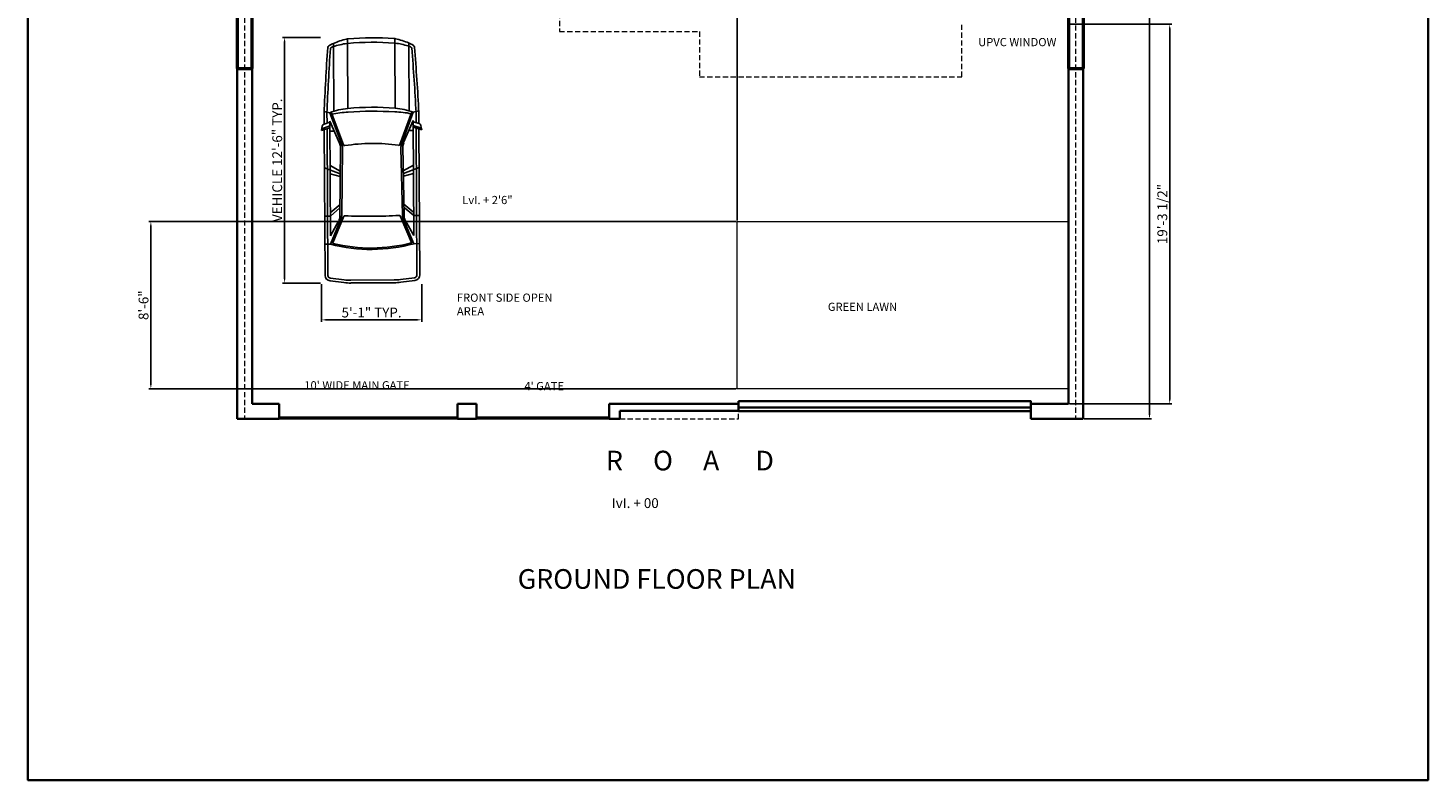
# Model space of a CAD drawing. Units: inches. Extents: x 2123 to 2977, y 1464 to 2698.
# Tile 1 of 10: x 2123 to 2977, y 1464 to 1923. Entities that reach past the tile are written whole.
import ezdxf

# ---------------------------------------------------------------- set-up
doc = ezdxf.new("R2010")
doc.units = ezdxf.units.IN
doc.linetypes.add('HIDDEN2', pattern=[4.7625, 3.175, -1.5875])
doc.layers.add('0 finos', color=250, linetype='Continuous')
for name, color, linetype, lineweight in [('A-ANNO-DIMS', 2, 'Continuous', 18), ('A-ANNO-SYMB', 7, 'Continuous', 18), ('A-ANNO-TEXT', 7, 'Continuous', 18), ('A-ANNO-TTLB', 7, 'Continuous', 35), ('A-AREA-IDEN', 7, 'Continuous', 25), ('A-FLOR-OVHD', 253, 'HIDDEN2', 18), ('A-WALL', 7, 'Continuous', 50), ('C-PKNG-VEHC', 8, 'Continuous', 18), ('C-PROP', 21, 'HIDDEN2', 18), ('L-PLNT-TURF', 3, 'Continuous', 18), ('L-SITE-GATE', 4, 'Continuous', 25), ('L-SITE-WALL', 7, 'Continuous', 35), ('L-SITE-WALL-HIDN', 253, 'HIDDEN2', 18)]:
    doc.layers.add(name, color=color, linetype=linetype, lineweight=lineweight)
doc.styles.get("Standard").update_dxf_attribs({"font": 'arial.ttf'})
doc.dimstyles.new('ISO-25', dxfattribs={"dimtxt": 6, "dimasz": 2.5, "dimexe": 1.25, "dimexo": 0.625, "dimtad": 1, "dimdec": 0, "dimlunit": 3, "dimtxsty": 'Standard', "dimcen": 2.5, "dimadec": 0, "dimazin": 0, "dimtfac": 1, "dimtdec": 0, "dimtmove": 0, "dimatfit": 3, "dimfxl": 1, "dimarcsym": 0})

# ---------------------------------------------------------------- blocks, each defined once
blk = doc.blocks.new('carro')
at = {"layer": '0 finos'}
for p, q in [((-1.274, 0.841), (-1.249, 0.743)), ((-1.246, 0.843), (-1.047, 0.844)), ((-1.246, 0.793), (-1.063, 0.794)), ((-1.099, 0.744), (0.965, 0.756)), ((-1.045, 0.847), (-1.079, 0.744)), ((-0.964, 0.889), (-1.011, 0.744)), ((-0.93, 0.895), (-1.007, 0.881)), ((-0.93, 0.895), (-0.979, 0.744)), ((-0.963, 0.794), (1.676, 0.81)), ((-0.947, 0.845), (1.676, 0.86)), ((-0.258, 0.849), (-0.148, 0.566)), ((0.61, 0.754), (0.609, 0.854)), ((0.669, 0.564), (1.115, 0.756)), ((0.701, 0.605), (0.965, 0.756)), ((0.965, 0.756), (0.778, 0.755)), ((1.115, 0.756), (1.114, 0.856)), ((1.759, 0.516), (1.726, 0.766)), ((1.809, 0.522), (1.776, 0.773)), ((-2.494, 0.661), (-2.439, 0.661)), ((-2.439, 0.661), (-1.275, 0.668)), ((-0.666, 0.502), (-1.258, 0.718)), ((-0.674, 0.532), (-1.249, 0.743)), ((-1.099, 0.744), (-0.702, 0.571)), ((-0.919, 0.745), (-0.919, 0.665)), ((0.615, 0.581), (-0.626, 0.557)), ((-0.608, 0.521), (0.602, 0.549)), ((-0.299, 0.748), (-0.198, 0.565)), ((-0.149, 0.749), (-0.098, 0.567)), ((0.551, 0.753), (0.402, 0.577)), ((0.61, 0.754), (0.462, 0.578)), ((0.616, 0.508), (1.094, 0.714)), ((-2.573, 0.41), (-2.493, 0.411)), ((-2.476, 0.411), (-1.323, 0.417)), ((1.771, -0.377), (1.767, 0.398)), ((1.821, -0.377), (1.817, 0.398)), ((-2.568, -0.44), (-2.488, -0.439)), ((-2.471, -0.439), (-1.318, -0.433)), ((1.102, -0.701), (0.622, -0.501)), ((1.765, -0.495), (1.735, -0.746)), ((1.814, -0.501), (1.785, -0.752)), ((-2.487, -0.689), (-2.432, -0.689)), ((-2.432, -0.689), (-1.267, -0.682)), ((-0.661, -0.51), (-1.25, -0.733)), ((-0.668, -0.54), (-1.241, -0.757)), ((-1.091, -0.756), (-0.695, -0.579)), ((-1.091, -0.756), (0.974, -0.744)), ((-0.911, -0.755), (-0.911, -0.676)), ((0.622, -0.574), (-0.62, -0.564)), ((-0.602, -0.528), (0.608, -0.542)), ((-0.291, -0.752), (-0.192, -0.567)), ((-0.248, -0.851), (-0.142, -0.568)), ((-0.141, -0.751), (-0.092, -0.568)), ((0.559, -0.747), (0.408, -0.572)), ((0.619, -0.746), (0.468, -0.573)), ((0.619, -0.746), (0.619, -0.846)), ((1.124, -0.743), (0.676, -0.556)), ((0.708, -0.597), (0.974, -0.744)), ((0.974, -0.744), (0.819, -0.745)), ((1.124, -0.843), (1.124, -0.743)), ((-1.262, -0.856), (-1.241, -0.757)), ((-1.237, -0.807), (-1.054, -0.806)), ((-1.236, -0.857), (-1.037, -0.856)), ((-1.036, -0.859), (-1.071, -0.756)), ((-0.953, -0.9), (-1.002, -0.756)), ((-0.92, -0.905), (-0.996, -0.892)), ((-0.92, -0.905), (-0.971, -0.756)), ((-0.954, -0.806), (1.686, -0.79)), ((-0.937, -0.855), (1.686, -0.84))]:
    blk.add_line(p, q, dxfattribs=at)
for centre, radius, start, end in [((-2.414, 0.72), 0.045, 99.6056, 145.8602), ((0.535, -34.533), 35.421, 92.8817, 94.7876), ((0.535, -34.583), 35.421, 92.8817, 94.7595), ((-0.998, 0.832), 0.05, 100.189, 161.8979), ((-2.008, -0.06), 3.228, 1.1964, 14.6587), ((1.677, 0.76), 0.1, 7.4579, 90.3329), ((1.677, 0.76), 0.05, 7.4579, 90.3329), ((-1.339, 0.159), 1.259, 156.5474, 167.8615), ((-2.14, 0.534), 0.376, 145.8602, 160.2963), ((-0.601, 0.138), 1.911, 164.4728, 171.5741), ((-2.25, 0.596), 0.2, 150.5092, 164.4728), ((-2.14, 0.534), 0.326, 147.5998, 150.5092), ((-2.403, 0.7), 0.015, 94.7595, 147.5998), ((-0.078, 0.306), 1.25, 159.5351, 174.8753), ((-0.049, 0.42), 1.205, 166.3495, 180.3763), ((-0.63, 0.737), 0.18, 246.5804, 271.1487), ((-0.612, 0.701), 0.18, 249.9002, 271.3224), ((0.598, 0.729), 0.18, 271.3224, 293.3542), ((0.622, 0.494), 0.015, 113.3542, 183.6852), ((0.612, 0.761), 0.18, 271.1487, 299.704), ((1.096, 0.709), 0.005, 13.9297, 113.3542), ((-2.008, -0.06), 3.203, 1.1964, 13.9297), ((0.817, 0.392), 0.95, 0.3329, 7.4579), ((0.817, 0.392), 1, 0.3329, 7.4579), ((2.688, 0.016), 5.275, 175.8587, 184.807), ((-2.375, 0.382), 0.2, 167.8615, 175.8587), ((2.688, 0.016), 5.195, 175.7191, 184.9467), ((-2.294, 0.389), 0.2, 171.5741, 175.7191), ((3.848, 0.022), 5.186, 175.6321, 185.0337), ((3.848, 0.022), 5.116, 175.6321, 185.0337), ((2.517, 0.015), 3.205, 171.6477, 189.0181), ((-0.673, 0.483), 0.02, 351.6477, 69.9002), ((-5.6, 0.093), 6.22, 359.1748, 3.6852), ((-5.599, -0.158), 6.22, 356.9806, 1.4909), ((-2.008, 0.037), 3.203, 346.7361, 359.4694), ((-2.008, 0.037), 3.228, 346.0071, 359.4694), ((-2.37, -0.41), 0.2, 184.807, 192.8043), ((-1.337, -0.175), 1.259, 192.8043, 204.1184), ((-2.289, -0.415), 0.2, 184.9467, 189.0917), ((-0.6, -0.145), 1.911, 189.0917, 196.7185), ((-0.074, -0.307), 1.25, 185.7904, 201.1307), ((-0.044, -0.42), 1.205, 180.2895, 194.3163), ((-0.668, -0.491), 0.02, 290.7656, 9.0181), ((0.628, -0.487), 0.015, 176.9806, 247.3115), ((0.822, -0.383), 0.95, 353.2079, 0.3329), ((0.822, -0.383), 1, 353.2079, 0.3329), ((-2.134, -0.558), 0.376, 200.3694, 214.8056), ((-2.406, -0.687), 0.025, 196.7185, 205.3192), ((-2.134, -0.558), 0.326, 205.3192, 213.066), ((-2.395, -0.728), 0.015, 213.066, 265.9063), ((0.133, 34.587), 35.421, 265.9063, 267.7841), ((-0.621, -0.744), 0.18, 89.5171, 114.0853), ((-0.604, -0.708), 0.18, 89.3433, 110.7656), ((0.606, -0.722), 0.18, 67.3115, 89.3433), ((0.621, -0.754), 0.18, 60.9617, 89.5171), ((1.104, -0.697), 0.005, 247.3115, 346.7361), ((1.685, -0.74), 0.05, 270.3329, 353.2079), ((1.685, -0.74), 0.1, 270.3329, 353.2079), ((-2.406, -0.748), 0.045, 214.8056, 261.0602), ((0.133, 34.537), 35.421, 265.8782, 267.7841), ((-0.988, -0.843), 0.05, 198.7678, 260.4768)]:
    blk.add_arc(centre, radius, start, end, dxfattribs=at)
blk = doc.blocks.new('*D9')
at = {"layer": 'A-ANNO-DIMS', "color": 0, "lineweight": -2, "transparency": 16777216}
for p, q in [((2767.56, 2548.37), (2808.58, 2548.37)), ((2807.33, 2545.87), (2807.33, 1686.46)), ((2767.56, 1683.96), (2808.58, 1683.96))]:
    blk.add_line(p, q, dxfattribs=at)
at = {"layer": 'A-ANNO-DIMS', "color": 0, "transparency": 16777216}
for points in [[(2806.91, 2545.87), (2807.74, 2545.87), (2807.33, 2548.37)], [(2806.91, 1686.46), (2807.74, 1686.46), (2807.33, 1683.96)]]:
    blk.add_solid(points, dxfattribs=at)
at = {"layer": 'Defpoints', "color": 0, "transparency": 16777216}
for p in [(2766.94, 2548.37), (2766.94, 1683.96), (2807.33, 1683.96)]:
    blk.add_point(p, dxfattribs=at)
at = {"layer": 'A-ANNO-DIMS', "color": 0, "transparency": 16777216, "insert": (2803.69, 2116.16), "char_height": 6, "attachment_point": 5, "rotation": 90}
blk.add_mtext("72'", dxfattribs=at)
blk = doc.blocks.new('*D40')
at = {"layer": 'A-ANNO-DIMS', "color": 0, "lineweight": -2, "transparency": 16777216}
for p, q in [((2301.67, 1916.86), (2278.56, 1916.86)), ((2279.81, 1914.36), (2279.81, 1769.44)), ((2301.67, 1766.94), (2278.56, 1766.94))]:
    blk.add_line(p, q, dxfattribs=at)
at = {"layer": 'A-ANNO-DIMS', "color": 0, "transparency": 16777216}
for points in [[(2279.39, 1914.36), (2280.23, 1914.36), (2279.81, 1916.86)], [(2279.39, 1769.44), (2280.23, 1769.44), (2279.81, 1766.94)]]:
    blk.add_solid(points, dxfattribs=at)
at = {"layer": 'Defpoints', "color": 0, "transparency": 16777216}
for p in [(2302.3, 1916.86), (2279.81, 1766.94), (2302.3, 1766.94)]:
    blk.add_point(p, dxfattribs=at)
at = {"layer": 'A-ANNO-DIMS', "color": 0, "transparency": 16777216, "insert": (2276.08, 1841.9), "char_height": 6, "attachment_point": 5, "rotation": 90}
blk.add_mtext('VEHICLE 12\'-6" TYP.', dxfattribs=at)
blk = doc.blocks.new('*D41')
at = {"layer": 'A-ANNO-DIMS', "color": 0, "lineweight": -2, "transparency": 16777216}
for p, q in [((2302.3, 1766.32), (2302.3, 1743.21)), ((2363.41, 1766.32), (2363.41, 1743.21)), ((2304.8, 1744.46), (2360.91, 1744.46))]:
    blk.add_line(p, q, dxfattribs=at)
at = {"layer": 'A-ANNO-DIMS', "color": 0, "transparency": 16777216}
for points in [[(2304.8, 1744.87), (2304.8, 1744.04), (2302.3, 1744.46)], [(2360.91, 1744.87), (2360.91, 1744.04), (2363.41, 1744.46)]]:
    blk.add_solid(points, dxfattribs=at)
at = {"layer": 'Defpoints', "color": 0, "transparency": 16777216}
for p in [(2302.3, 1766.94), (2363.41, 1766.94), (2363.41, 1744.46)]:
    blk.add_point(p, dxfattribs=at)
at = {"layer": 'A-ANNO-DIMS', "color": 0, "transparency": 16777216, "insert": (2332.85, 1748.14), "char_height": 6, "attachment_point": 5}
blk.add_mtext('5\'-1" TYP.', dxfattribs=at)
blk = doc.blocks.new('*D55')
at = {"layer": 'A-ANNO-DIMS', "color": 0, "lineweight": -2, "transparency": 16777216}
for p, q in [((2758.56, 1924.87), (2820.89, 1924.87)), ((2819.64, 1695.76), (2819.64, 1922.37)), ((2758.56, 1693.26), (2820.89, 1693.26))]:
    blk.add_line(p, q, dxfattribs=at)
at = {"layer": 'A-ANNO-DIMS', "color": 0, "transparency": 16777216}
for points in [[(2819.22, 1922.37), (2820.05, 1922.37), (2819.64, 1924.87)], [(2819.22, 1695.76), (2820.05, 1695.76), (2819.64, 1693.26)]]:
    blk.add_solid(points, dxfattribs=at)
at = {"layer": 'Defpoints', "color": 0, "transparency": 16777216}
for p in [(2757.94, 1924.87), (2819.64, 1924.87), (2757.94, 1693.26)]:
    blk.add_point(p, dxfattribs=at)
at = {"layer": 'A-ANNO-DIMS', "color": 0, "transparency": 16777216, "insert": (2815.91, 1809.06), "char_height": 6, "attachment_point": 5, "rotation": 90}
blk.add_mtext('19\'-3 1/2"', dxfattribs=at)
blk = doc.blocks.new('*D57')
at = {"layer": 'A-ANNO-DIMS', "color": 0, "lineweight": -2, "transparency": 16777216}
for p, q in [((2555.89, 1805.13), (2555.89, 2606.82)), ((2558.39, 2605.57), (2755.44, 2605.57)), ((2757.94, 1805.13), (2757.94, 2606.82))]:
    blk.add_line(p, q, dxfattribs=at)
at = {"layer": 'A-ANNO-DIMS', "color": 0, "transparency": 16777216}
for points in [[(2558.39, 2605.99), (2558.39, 2605.15), (2555.89, 2605.57)], [(2755.44, 2605.99), (2755.44, 2605.15), (2757.94, 2605.57)]]:
    blk.add_solid(points, dxfattribs=at)
at = {"layer": 'Defpoints', "color": 0, "transparency": 16777216}
for p in [(2757.94, 2605.57), (2555.89, 1804.5), (2757.94, 1804.5)]:
    blk.add_point(p, dxfattribs=at)
at = {"layer": 'A-ANNO-DIMS', "color": 0, "transparency": 16777216, "insert": (2656.91, 2609.26), "char_height": 6, "attachment_point": 5}
blk.add_mtext('16\'-10"', dxfattribs=at)
blk = doc.blocks.new('*D58')
at = {"layer": 'A-ANNO-DIMS', "color": 0, "lineweight": -2, "transparency": 16777216}
for p, q in [((2555.26, 1804.5), (2196.99, 1804.5)), ((2198.24, 1704.8), (2198.24, 1802)), ((2555.26, 1702.3), (2196.99, 1702.3))]:
    blk.add_line(p, q, dxfattribs=at)
at = {"layer": 'A-ANNO-DIMS', "color": 0, "transparency": 16777216}
for points in [[(2197.82, 1802), (2198.65, 1802), (2198.24, 1804.5)], [(2197.82, 1704.8), (2198.65, 1704.8), (2198.24, 1702.3)]]:
    blk.add_solid(points, dxfattribs=at)
at = {"layer": 'Defpoints', "color": 0, "transparency": 16777216}
for p in [(2198.24, 1804.5), (2555.89, 1804.5), (2555.89, 1702.3)]:
    blk.add_point(p, dxfattribs=at)
at = {"layer": 'A-ANNO-DIMS', "color": 0, "transparency": 16777216, "insert": (2194.55, 1753.4), "char_height": 6, "attachment_point": 5, "rotation": 90}
blk.add_mtext('8\'-6"', dxfattribs=at)

msp = doc.modelspace()

# ---------------------------------------------------------------- linework, layer by layer
at = {"layer": 'A-ANNO-SYMB'}
msp.add_line((2486.66, 1632.88), (2486.66, 1632.88), dxfattribs=at)
at = {"layer": 'A-ANNO-TTLB'}
msp.add_lwpolyline([(2123.3, 2697.62), (2977.18, 2697.62), (2977.18, 1463.53), (2123.3, 1463.53)], close=True, dxfattribs=at)
at = {"layer": 'A-FLOR-OVHD'}
for p, q in [((2447.44, 1969.87), (2447.44, 1920.38)), ((2692.84, 1892.82), (2692.84, 1924.87)), ((2447.44, 1920.38), (2532.81, 1920.38)), ((2532.81, 1920.38), (2532.81, 1892.82)), ((2532.81, 1892.82), (2692.84, 1892.82))]:
    msp.add_line(p, q, dxfattribs=at)
at = {"layer": 'A-WALL'}
for p, q in [((2766.94, 2425.87), (2766.94, 1897.87)), ((2757.94, 2416.87), (2757.94, 1897.87)), ((2250.94, 1969.87), (2250.94, 1909.87)), ((2259.94, 1897.87), (2259.94, 1969.87)), ((2250.94, 1909.87), (2250.94, 1897.87)), ((2250.94, 1897.87), (2259.94, 1897.87)), ((2757.94, 1897.87), (2766.94, 1897.87))]:
    msp.add_line(p, q, dxfattribs=at)
at = {"layer": 'C-PROP'}
for p, q in [((2255.34, 2552.87), (2255.44, 1683.96)), ((2762.16, 2552.87), (2762.16, 1683.96)), ((2762.16, 1683.96), (2762.16, 1683.96))]:
    msp.add_line(p, q, dxfattribs=at)
at = {"layer": 'L-PLNT-TURF'}
msp.add_lwpolyline([(2555.89, 1804.5), (2757.94, 1804.5), (2757.94, 1702.3), (2555.89, 1702.3)], close=True, dxfattribs=at)
at = {"layer": 'L-SITE-GATE'}
for p, q in [((2276.55, 1685.11), (2385.28, 1685.11)), ((2276.55, 1683.96), (2477.69, 1683.96)), ((2396.77, 1685.11), (2477.69, 1685.11))]:
    msp.add_line(p, q, dxfattribs=at)
at = {"layer": 'L-SITE-WALL'}
for p, q in [((2250.94, 1897.87), (2250.94, 1683.96)), ((2259.94, 1693.26), (2259.94, 1897.87)), ((2757.94, 1897.87), (2757.94, 1693.26)), ((2766.94, 1897.87), (2766.94, 1687.09)), ((2259.94, 1693.26), (2276.55, 1693.26)), ((2276.55, 1693.26), (2276.55, 1683.96)), ((2385.28, 1683.96), (2385.28, 1693.26)), ((2385.28, 1693.26), (2396.77, 1693.26)), ((2396.77, 1693.26), (2396.77, 1683.96)), ((2477.69, 1693.26), (2556.7, 1693.26)), ((2477.69, 1693.26), (2477.69, 1683.96)), ((2556.7, 1688.82), (2556.7, 1693.26)), ((2556.7, 1691.04), (2735.01, 1691.04)), ((2735.01, 1693.26), (2735.01, 1683.96)), ((2757.94, 1693.26), (2735.01, 1693.26)), ((2735.01, 1691.04), (2735.01, 1690.77)), ((2250.94, 1683.96), (2259.94, 1683.96)), ((2259.94, 1683.96), (2276.55, 1683.96)), ((2396.77, 1683.96), (2385.28, 1683.96)), ((2477.69, 1683.96), (2484.26, 1683.96)), ((2484.26, 1683.96), (2484.26, 1688.82)), ((2484.26, 1688.82), (2556.7, 1688.82)), ((2766.94, 1683.96), (2735.01, 1683.96)), ((2766.94, 1683.96), (2766.94, 1687.09))]:
    msp.add_line(p, q, dxfattribs=at)
msp.add_lwpolyline([(2556.7, 1694.75), (2735.01, 1694.75), (2735.01, 1688.61), (2556.7, 1688.61)], close=True, dxfattribs=at)
at = {"layer": 'L-SITE-WALL-HIDN'}
for p, q in [((2484.26, 1683.96), (2556.7, 1683.96)), ((2556.7, 1683.96), (2556.7, 1688.82))]:
    msp.add_line(p, q, dxfattribs=at)

# ---------------------------------------------------------------- block references
at = {"layer": 'C-PKNG-VEHC', "xscale": 33.95074894597202, "yscale": 33.95074894597202, "zscale": 33.95074894597202, "rotation": 270}
msp.add_blockref('carro', (2333.04, 1828.79), dxfattribs=at)

# ---------------------------------------------------------------- texts
at = {"layer": 'A-ANNO-SYMB', "attachment_point": 1}
for s, width, insert, char_height in [('LvI. + 2\'6"', 307.2899, (2388.16, 1820.11), 5), ('IvI. + 00', 173.0019, (2479.36, 1635.58), 6)]:
    msp.add_mtext_dynamic_manual_height_columns(s, width=width, gutter_width=12.5, heights=[0], dxfattribs=dict(at, insert=insert, char_height=char_height))
at = {"layer": 'A-ANNO-TEXT', "char_height": 5, "attachment_point": 1}
for s, width, insert in [('UPVC WINDOW', 103.2245, (2702.83, 1916.5)), ("10' WIDE MAIN GATE", 284.3741, (2291.83, 1707.01)), ("4' GATE", 186.8996, (2426.07, 1706.52))]:
    msp.add_mtext_dynamic_manual_height_columns(s, width=width, gutter_width=12.5, heights=[0], dxfattribs=dict(at, insert=insert))
at = {"layer": 'A-ANNO-TTLB', "insert": (2421.97, 1592.27), "char_height": 12, "attachment_point": 1}
msp.add_mtext_dynamic_manual_height_columns('GROUND FLOOR PLAN', width=458.4396, gutter_width=12.5, heights=[0], dxfattribs=at)
at = {"layer": 'A-AREA-IDEN', "attachment_point": 1}
for s, width, insert, char_height in [('FRONT SIDE OPEN \\PAREA', 237.5857, (2384.88, 1760.5), 5), ('GREEN LAWN', 678.6839, (2611.12, 1754.91), 5), ('R     O     A      D', 574.0394, (2475.8, 1664.54), 12)]:
    msp.add_mtext_dynamic_manual_height_columns(s, width=width, gutter_width=12.5, heights=[0], dxfattribs=dict(at, insert=insert, char_height=char_height))

# ---------------------------------------------------------------- dimensions: what is measured, and where the dimension line sits
at = {"layer": 'A-ANNO-DIMS'}
dim = msp.add_linear_dim(base=(2757.9353, 2605.5708), p1=(2555.8869, 1804.5032), p2=(2757.9353, 1804.5032), dimstyle='ISO-25', override={"dimdec": 1, "dimlfac": 1, "dimrnd": 0, "dimzin": 1, "dimdsep": 46, "dimlunit": 4, "dimfrac": 2}, dxfattribs=at)
dim.commit()
dim.dimension.update_dxf_attribs({"geometry": '*D57', "text_midpoint": (2656.9111, 2609.2592)})
for base, p1, p2, override, picture, middle in [((2807.33, 1683.96), (2766.94, 2548.37), (2766.94, 1683.96), {"dimclrd": 0, "dimclre": 0, "dimclrt": 0}, '*D9', (2803.69, 2116.16)), ((2819.64, 1924.87), (2757.94, 1693.26), (2757.94, 1924.87), {"dimdec": 1, "dimlfac": 1, "dimrnd": 0, "dimzin": 1, "dimdsep": 46, "dimlunit": 4, "dimfrac": 2}, '*D55', (2815.91, 1809.06)), ((2198.24, 1804.5), (2555.89, 1702.3), (2555.89, 1804.5), {"dimdec": 1, "dimlfac": 1, "dimrnd": 0, "dimzin": 1, "dimdsep": 46, "dimlunit": 4, "dimfrac": 2}, '*D58', (2194.55, 1753.4))]:
    dim = msp.add_linear_dim(base=base, p1=p1, p2=p2, angle=90, dimstyle='ISO-25', override=override, dxfattribs=at)
    dim.commit()
    dim.dimension.update_dxf_attribs({"geometry": picture, "text_midpoint": middle})
dim = msp.add_linear_dim(base=(2279.81, 1766.94), p1=(2302.3, 1916.86), p2=(2302.3, 1766.94), angle=270, text='VEHICLE <> TYP.', dimstyle='ISO-25', override={"dimdec": 1, "dimlfac": 1, "dimrnd": 0, "dimzin": 1, "dimdsep": 46, "dimlunit": 4, "dimfrac": 2}, dxfattribs=at)
dim.commit()
dim.dimension.update_dxf_attribs({"geometry": '*D40', "text_midpoint": (2276.08, 1841.9)})
dim = msp.add_linear_dim(base=(2363.41, 1744.46), p1=(2302.3, 1766.94), p2=(2363.41, 1766.94), text='<> TYP.', dimstyle='ISO-25', override={"dimdec": 1, "dimlfac": 1, "dimrnd": 0, "dimzin": 1, "dimdsep": 46, "dimlunit": 4, "dimfrac": 2}, dxfattribs=at)
dim.commit()
dim.dimension.update_dxf_attribs({"geometry": '*D41', "text_midpoint": (2332.85, 1748.14)})

doc.saveas('drawing.dxf')
